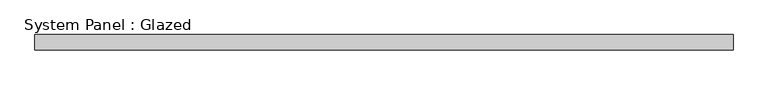
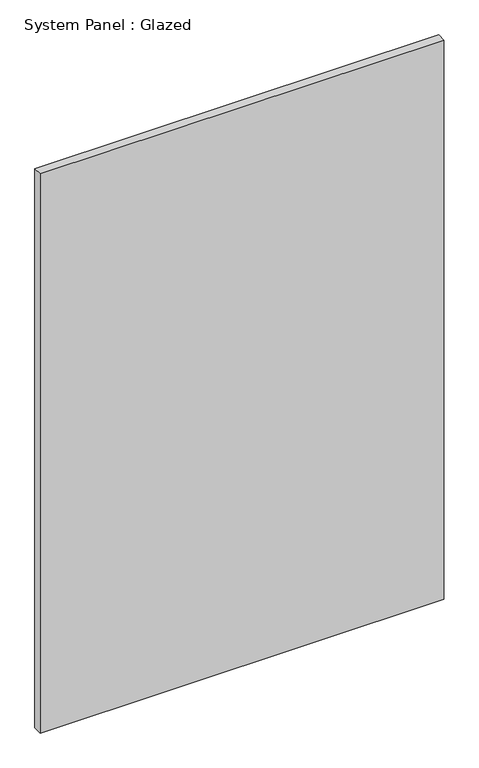
"""IFC4 building model written with IfcOpenShell, lengths in millimetres: plate geometry, System Panel : Glazed."""

from ifc_helpers import new_model, si_unit, origin, origin_with_axes, place, context, project, spatial, polyline, outline, extrude, source, transform, mapped, element, save


def system_panel_glazed_da159ad5(model_context):
    return source(origin(), model_context, "Body", "SweptSolid", [
        extrude(outline(polyline([(577.7496112, 19.05), (-577.7496112, 19.05), (-577.7496112, 44.45), (577.7496112, 44.45), (577.7496112, 19.05)])), origin_with_axes(), (0.0, 0.0, 1.0), 1691.9879691),
    ])


if __name__ == "__main__":
    model = new_model("IFC4")
    model_context = context("Model", 3, world=origin())
    ifc_project = project(units=[si_unit("LENGTHUNIT", "METRE", prefix="MILLI")], contexts=[model_context])
    site = spatial("IfcSite", under=ifc_project)
    building = spatial("IfcBuilding", under=site)
    placement = place(None, origin())
    system_panel_glazed_shape = system_panel_glazed_da159ad5(model_context)
    element("IfcPlate", 1, ObjectType="System Panel : Glazed", at=placement, inside=building, context=model_context, shape_type="MappedRepresentation", body=[
        mapped(system_panel_glazed_shape, transform((0.0, 0.0, 0.0), x_axis=(1.0, 0.0, 0.0), y_axis=(0.0, 1.0, 0.0), z_axis=(0.0, 0.0, 1.0))),
    ])
    save(model, "model.ifc")

# Revit data of these elements
# Type "System Panel : Glazed"
#   Construction Type Id = "GSP4R"
#   Analytic Construction = "1/8 in Pilkington single glazing"
#   Visual Light Transmittance = 0.9
#   Solar Heat Gain Coefficient = 0.86
#   Heat Transfer Coefficient (U) = 1.18115 BTU/(h·ft²·°F)
#   Define Thermal Properties by = 1
# Element 1 (IfcPlate, "System Panel : Glazed")
#   Materials on its faces: "Glass"
# Materials
#   "Glass": class "Glass", colour RGB 0 128 192, transparency 0.75, Description = "Soda Lime Glass", Cost = 0
